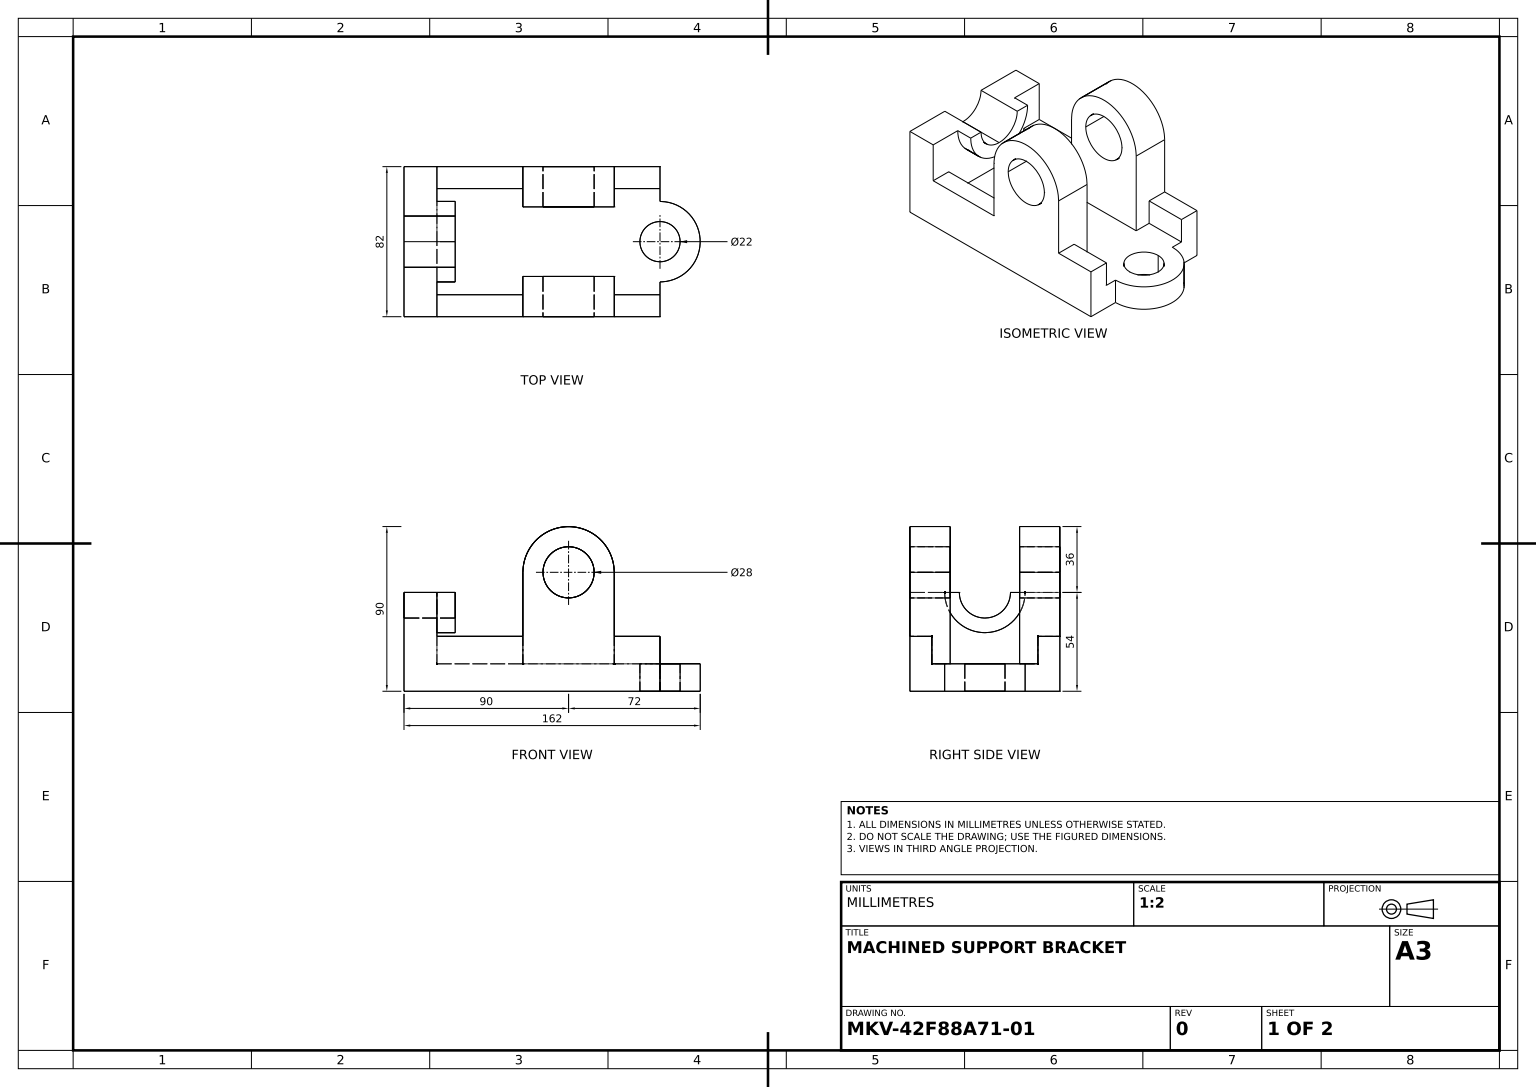
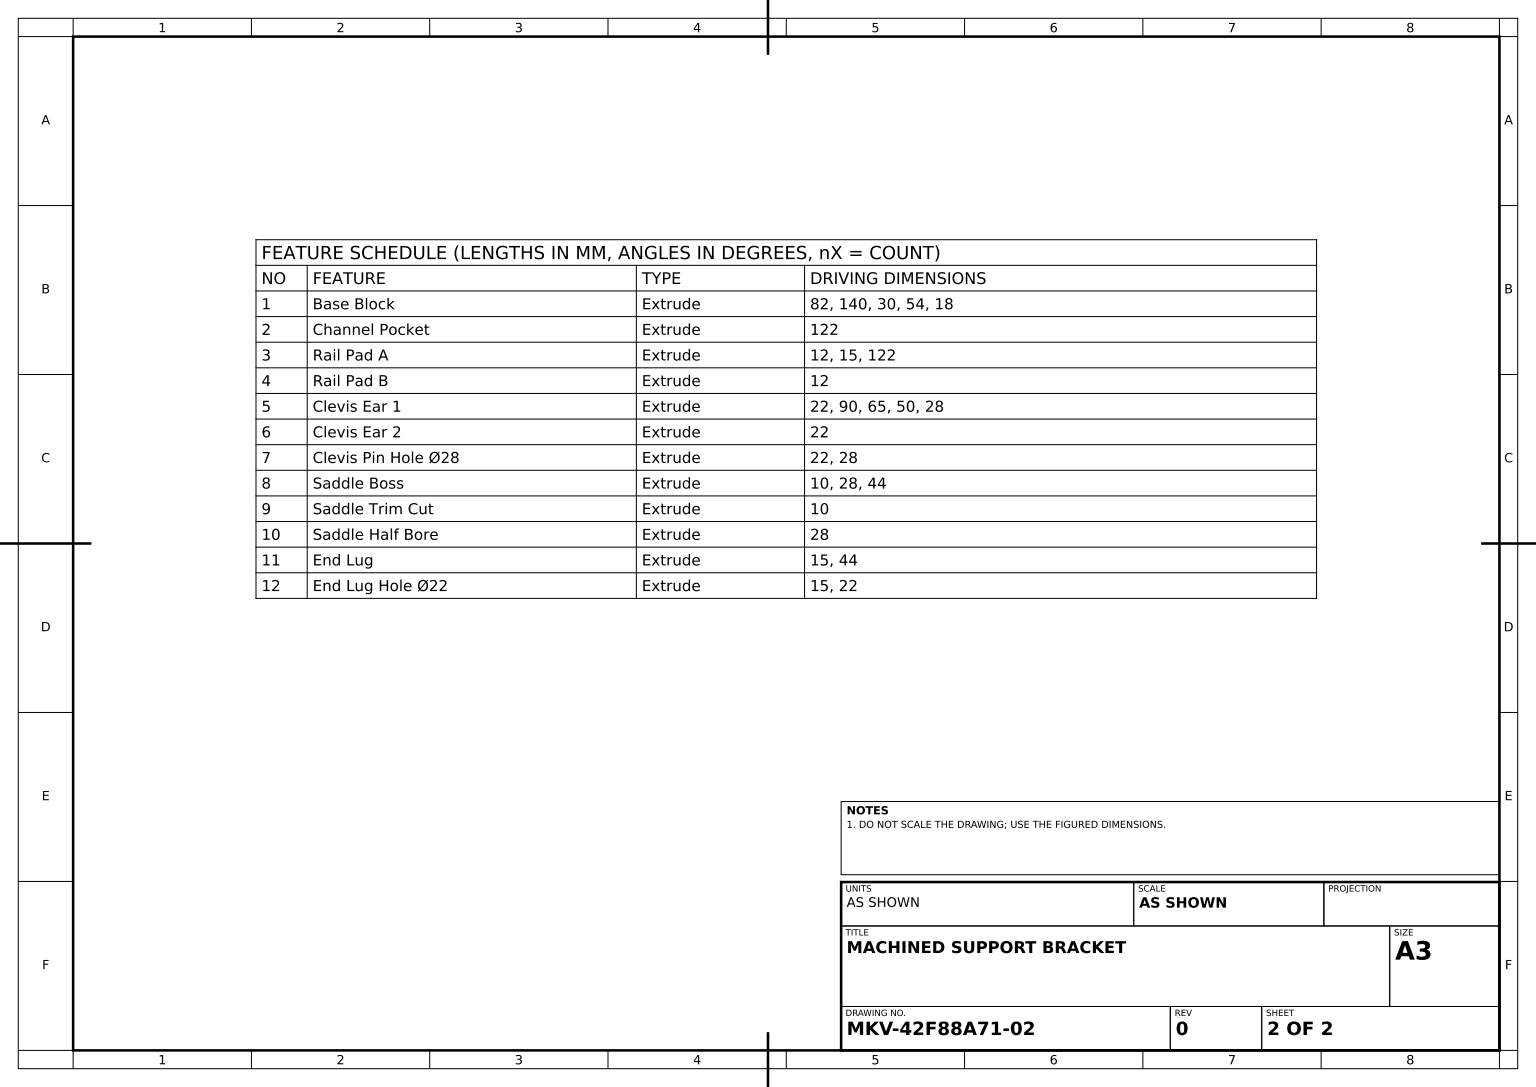
from build123d import *

# Parameters (mm, degrees)
BASE_BLOCK_DEPTH         = 41
CHANNEL_POCKET_SKETCH_W  = 82
CHANNEL_POCKET_SKETCH_H  = 15
CHANNEL_POCKET_DEPTH     = 122
RAIL_PAD_A_SKETCH_W      = 122
RAIL_PAD_A_SKETCH_H      = 15
RAIL_PAD_A_DEPTH         = 12
RAIL_PAD_B_SKETCH_W      = 122
RAIL_PAD_B_SKETCH_H      = 15
RAIL_PAD_B_DEPTH         = 12
CLEVIS_EAR_1_SKETCH_R    = 14
CLEVIS_EAR_1_DEPTH       = 22
CLEVIS_START             = -22
CLEVIS_EAR_2_SKETCH_W    = 50
CLEVIS_EAR_2_SKETCH_H    = 15
CLEVIS_EAR_2_DEPTH       = 22
CLEVIS_PIN_HOLE_SKETCH_R = 14
CLEVIS_PIN_HOLE_28_DEPTH = 22
SADDLE_BOSS_SKETCH_R     = 22
SADDLE_BOSS_SKETCH_R_2   = 14
SADDLE_BOSS_DEPTH        = 10
SADDLE_START             = -10
SADDLE_TRIM_CUT_DEPTH    = 10
SADDLE_START_2           = -28
SADDLE_BORE_SKETCH_R     = 14
SADDLE_HALF_BORE_DEPTH   = 28
END_LUG_DEPTH            = 15
END_LUG_HOLE_SKETCH_R    = 11
END_LUG_HOLE_22_DEPTH    = 15


with BuildPart() as part:
    # Base Profile Sketch → Base Block (new, symmetric)
    with BuildSketch(Plane.XY):
        Polygon((0, 0), (0, 54), (18, 54), (18, 30), (140, 30), (140, 0), align=None)
    extrude(amount=BASE_BLOCK_DEPTH, both=True)

    # Channel Pocket Sketch → Channel Pocket (cut)
    with BuildSketch(Plane(origin=(140, 0, 0), x_dir=(0, 0, -1), z_dir=(1, 0, 0))):
        with Locations((0, 22.5)):
            Rectangle(CHANNEL_POCKET_SKETCH_W, CHANNEL_POCKET_SKETCH_H)
    extrude(amount=-CHANNEL_POCKET_DEPTH, mode=Mode.SUBTRACT)

    # Rail Pad A Sketch → Rail Pad A (add)
    with BuildSketch(Plane.XY.offset(41)):
        with Locations((79, 22.5)):
            Rectangle(RAIL_PAD_A_SKETCH_W, RAIL_PAD_A_SKETCH_H)
    extrude(amount=-RAIL_PAD_A_DEPTH)

    # Rail Pad B Sketch → Rail Pad B (add)
    with BuildSketch(Plane(origin=(0, 0, -41), x_dir=(-1, 0, 0), z_dir=(0, 0, -1))):
        with Locations((-79, 22.5)):
            Rectangle(RAIL_PAD_B_SKETCH_W, RAIL_PAD_B_SKETCH_H)
    extrude(amount=-RAIL_PAD_B_DEPTH)

    # Clevis Ear 1 Sketch → Clevis Ear 1 (add)
    with BuildSketch(Plane.XY.offset(41)):
        with BuildLine():
            Line((65, 65), (65, 15))
            Line((65, 15), (115, 15))
            Line((115, 15), (115, 65))
            ThreePointArc((115, 65), (90, 90), (65, 65))
        make_face()
        with Locations((90, 65)):
            Circle(CLEVIS_EAR_1_SKETCH_R, mode=Mode.SUBTRACT)
    extrude(amount=-CLEVIS_EAR_1_DEPTH)

    # Clevis Ear 2 Sketch → Clevis Ear 2 (add)
    with BuildSketch(Plane(origin=(0, 0, -41), x_dir=(-1, 0, 0), z_dir=(0, 0, -1)).offset(CLEVIS_START)):
        with BuildLine():
            Line((-115, 30), (-65, 30))
            Line((-65, 30), (-65, 65))
            ThreePointArc((-65, 65), (-90, 90), (-115, 65))
            Line((-115, 65), (-115, 30))
        make_face()
        with Locations((-90, 22.5)):
            Rectangle(CLEVIS_EAR_2_SKETCH_W, CLEVIS_EAR_2_SKETCH_H)
    extrude(amount=CLEVIS_EAR_2_DEPTH)

    # Clevis Pin Hole Sketch → Clevis Pin Hole Ø28 (cut)
    with BuildSketch(Plane(origin=(0, 0, -41), x_dir=(-1, 0, 0), z_dir=(0, 0, -1)).offset(CLEVIS_START)):
        with Locations(Location((-90, 65, 0), (0, 0, 180))):
            Circle(CLEVIS_PIN_HOLE_SKETCH_R)
    extrude(amount=CLEVIS_PIN_HOLE_28_DEPTH, mode=Mode.SUBTRACT)

    # Saddle Boss Sketch → Saddle Boss (add)
    with BuildSketch(Plane(origin=(18, 0, 0), x_dir=(0, 0, -1), z_dir=(1, 0, 0))):
        with Locations((0, 54)):
            Circle(SADDLE_BOSS_SKETCH_R)
        with Locations(Location((0, 54, 0), (0, 0, 180))):
            Circle(SADDLE_BOSS_SKETCH_R_2, mode=Mode.SUBTRACT)
    extrude(amount=SADDLE_BOSS_DEPTH)

    # Saddle Trim Sketch → Saddle Trim Cut (cut)
    with BuildSketch(Plane(origin=(28, 0, 0), x_dir=(0, 0, -1), z_dir=(1, 0, 0)).offset(SADDLE_START)):
        with BuildLine():
            ThreePointArc((22, 54), (0, 76), (-22, 54))
            Line((-22, 54), (-14, 54))
            ThreePointArc((-14, 54), (0, 68), (14, 54))
            Line((14, 54), (22, 54))
        make_face()
    extrude(amount=SADDLE_TRIM_CUT_DEPTH, mode=Mode.SUBTRACT)

    # Saddle Bore Sketch → Saddle Half Bore (cut)
    with BuildSketch(Plane(origin=(28, 0, 0), x_dir=(0, 0, -1), z_dir=(1, 0, 0)).offset(SADDLE_START_2)):
        with Locations((0, 54)):
            Circle(SADDLE_BORE_SKETCH_R)
    extrude(amount=SADDLE_HALF_BORE_DEPTH, mode=Mode.SUBTRACT)

    # End Lug Sketch → End Lug (add)
    with BuildSketch(Plane.XZ):
        with BuildLine():
            Line((140, 22), (140, -22))
            ThreePointArc((140, -22), (162, 0), (140, 22))
        make_face()
    extrude(amount=-END_LUG_DEPTH)

    # End Lug Hole Sketch → End Lug Hole Ø22 (cut)
    with BuildSketch(Plane.XZ):
        with Locations(Location((140, 0, 0), (0, 0, 270))):
            Circle(END_LUG_HOLE_SKETCH_R)
    extrude(amount=-END_LUG_HOLE_22_DEPTH, mode=Mode.SUBTRACT)


solid = part.part
